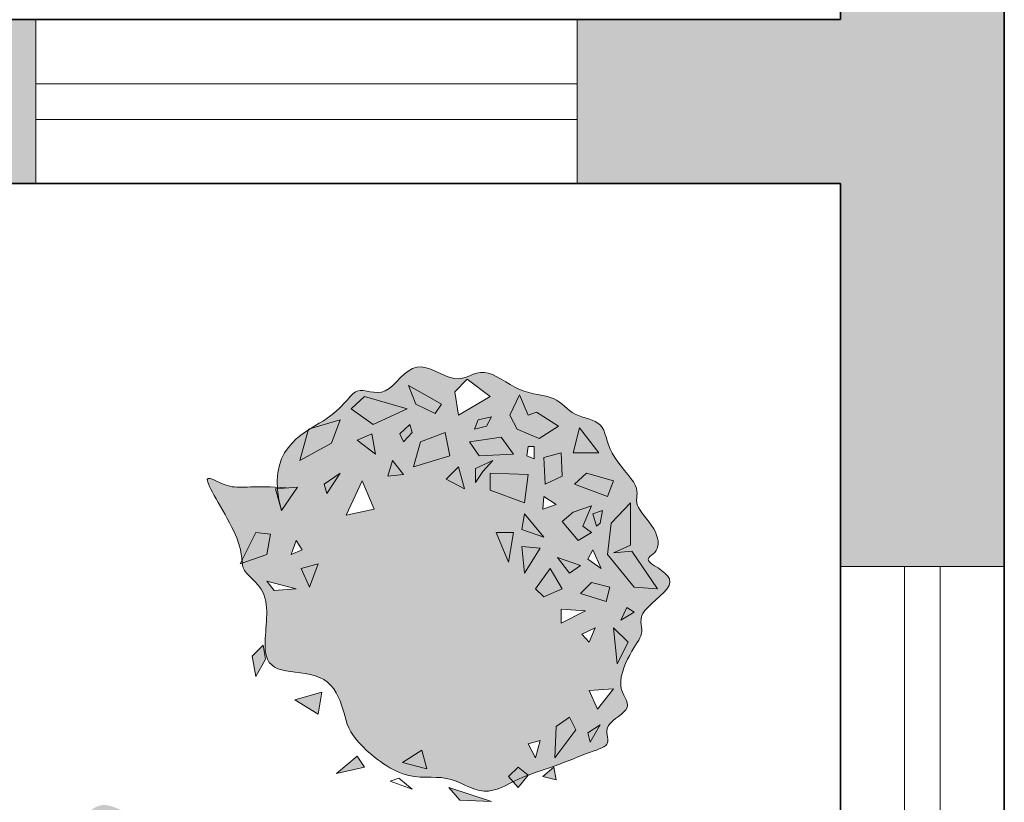
# Model space of a CAD drawing. Units: metres. Extents: x 4298.5 to 4325.2, y 2075 to 2095.8.
# Tile 15 of 35: x 4304.5 to 4305.9, y 2083.7 to 2084.8. Entities that reach past the tile are written whole.
import ezdxf

# ---------------------------------------------------------------- set-up
doc = ezdxf.new("R2010")
doc.units = ezdxf.units.M
for name, color, linetype, lineweight in [('A-ANNO-DIMS', 2, 'Continuous', 18), ('A-GLAZ', 4, 'Continuous', 18), ('A-WALL', 7, 'Continuous', 35), ('A-WALL-PATT', 252, 'Continuous', 13), ('L-PLNT', 94, 'Continuous', 13)]:
    doc.layers.add(name, color=color, linetype=linetype, lineweight=lineweight)
doc.layers.add('L-PLNT-PATT', color=116, linetype='Continuous', lineweight=13, true_color=0x13823e)
doc.styles.get("Standard").update_dxf_attribs({"font": 'arial.ttf'})
doc.dimstyles.get("Standard").update_dxf_attribs({"dimtxt": 0.18, "dimasz": 0.18, "dimexe": 0.18, "dimexo": 0.0625, "dimgap": 0.09, "dimtad": 0, "dimtih": 1, "dimtoh": 1, "dimdec": 4, "dimzin": 0, "dimdsep": 46, "dimtxsty": 'Standard', "dimcen": 0.09, "dimadec": 0, "dimazin": 0, "dimtfac": 1, "dimtdec": 4, "dimtofl": 0, "dimtmove": 0, "dimatfit": 3, "dimfxl": 1, "dimtolj": 1, "dimtzin": 0, "dimarcsym": 0})

# ---------------------------------------------------------------- blocks, each defined once
blk = doc.blocks.new('*U9')
for points in [[(1.237, 12.003), (0.562, 11.31), (0.764, 10.013), (2.519, 11.051)], [(-2.003, 11.656), (-1.598, 10.618), (-0.518, 10.099), (-0.181, 10.618), (-0.788, 10.964)], [(-4.432, 11.051), (-5.175, 10.359), (-3.96, 9.493), (-2.07, 10.359)], [(4.139, 11.137), (3.599, 10.013), (4.004, 9.234), (5.218, 8.715), (6.298, 9.407), (5.083, 10.186), (4.611, 10.013)], [(2.586, 9.926), (1.844, 9.753), (1.642, 9.234), (2.316, 9.407)], [(-5.782, 9.753), (-7.537, 9.234), (-8.009, 7.504), (-6.255, 8.455)], [(-1.935, 9.493), (-2.475, 8.974), (-2.273, 8.542), (-1.8, 9.061)], [(7.446, 9.32), (7.108, 7.936), (8.525, 7.936)], [(-4.837, 8.628), (-3.825, 7.85), (-4.027, 8.974)], [(0.022, 9.061), (-1.328, 8.542), (-1.733, 7.157), (0.292, 7.763)], [(1.372, 8.542), (3.126, 8.801), (3.801, 7.85), (1.912, 7.763)], [(4.611, 8.282), (4.544, 7.763), (4.949, 7.59), (4.949, 8.282)], [(6.433, 7.936), (5.488, 7.676), (5.556, 6.206), (6.501, 6.638)], [(-2.88, 7.504), (-3.15, 6.638), (-2.273, 6.725)], [(0.764, 7.157), (0.089, 6.465), (1.102, 5.946)], [(1.709, 6.292), (1.709, 7.071), (2.654, 7.504), (2.114, 6.898)], [(-5.782, 6.811), (-6.659, 6.206), (-6.524, 5.687)], [(2.519, 6.811), (2.519, 5.86), (4.409, 5.167), (4.611, 6.725)], [(7.851, 6.811), (7.176, 6.206), (8.998, 5.514), (9.335, 6.379)], [(-8.144, 6.033), (-9.359, 5.946), (-9.022, 4.735)], [(-4.567, 6.379), (-5.445, 4.475), (-3.892, 4.821)], [(5.488, 5.514), (5.421, 4.821), (6.163, 5.081)], [(8.12, 4.994), (7.108, 4.648), (6.501, 4.129), (7.378, 3.091), (8.12, 3.524), (7.648, 3.87)], [(10.28, 5.167), (9.2, 4.043), (8.998, 2.312), (10.482, 0.495), (11.765, 0.409), (10.348, 2.485), (9.335, 2.399), (10.28, 2.831)], [(4.409, 4.562), (4.274, 3.697), (5.488, 3.264)], [(8.728, 4.735), (8.188, 4.562), (8.39, 3.87), (8.593, 4.043)], [(-11.316, 1.793), (-9.831, 2.312), (-9.629, 3.437), (-10.439, 3.524)], [(3.531, 1.88), (2.856, 3.524), (3.801, 3.524)], [(-8.212, 3.091), (-8.482, 2.312), (-7.874, 2.572)], [(4.274, 2.745), (5.286, 2.658), (4.409, 1.274)], [(8.188, 2.572), (7.918, 2.053), (8.66, 1.534)], [(-6.997, 1.793), (-7.942, 1.534), (-7.469, 0.495)], [(7.513, 1.707), (6.906, 1.274), (6.231, 2.139)], [(5.826, 1.534), (5.016, 0.409), (5.488, -0.024), (6.501, 0.409)], [(-8.212, 0.409), (-9.426, 0.322), (-9.831, 0.841)], [(8.12, 0.755), (7.513, 0.149), (8.93, -0.283), (9.133, 0.495)], [(7.783, -0.803), (6.433, -1.495), (6.433, -0.716)], [(10.078, -0.629), (9.74, -1.322), (10.482, -0.889)], [(8.323, -1.754), (7.985, -2.533), (7.581, -2.1)], [(9.335, -1.754), (9.538, -3.744), (10.145, -2.533)], [(-10.034, -2.706), (-10.641, -3.312), (-10.439, -4.436), (-9.899, -3.485)], [(-8.279, -5.734), (-6.794, -5.302), (-6.997, -6.513)], [(9.335, -5.129), (8.458, -6.253), (7.985, -5.215)], [(6.096, -8.935), (6.163, -7.205), (6.906, -6.686), (7.243, -7.378)], [(8.053, -8.07), (8.593, -7.118), (7.918, -7.551)], [(5.286, -7.984), (4.611, -8.157), (5.016, -8.935)], [(-2.34, -9.195), (-1.26, -8.503), (-0.99, -9.541)], [(-4.837, -8.849), (-4.432, -9.454), (-5.985, -9.801)], [(4.071, -9.454), (3.531, -9.974), (4.071, -10.579), (4.611, -9.887)], [(6.028, -9.454), (5.421, -9.974), (6.163, -10.147)], [(-2.543, -10.06), (-3.015, -10.233), (-1.8, -10.666)], [(0.224, -10.579), (0.832, -11.272), (2.586, -11.358)]]:
    blk.add_lwpolyline(points, close=True)
blk = doc.blocks.new('WIN-760-GLASS')
for p, q in [((0, 0.76), (0, 0)), ((0.05, 0.76), (0.05, 0))]:
    blk.add_line(p, q)
blk = doc.blocks.new('*D47')
at = {"layer": 'A-ANNO-DIMS', "color": 0, "lineweight": -2, "transparency": 16777216}
for p, q in [((4300.4306, 2084.4956), (4300.4306, 2074.9896)), ((4322.8106, 2084.4956), (4322.8106, 2074.9896)), ((4300.6106, 2075.1696), (4311.2252, 2075.1696)), ((4322.6306, 2075.1696), (4312.016, 2075.1696))]:
    blk.add_line(p, q, dxfattribs=at)
at = {"layer": 'A-ANNO-DIMS', "color": 0, "transparency": 16777216}
for points in [[(4300.6106, 2075.1996), (4300.6106, 2075.1396), (4300.4306, 2075.1696)], [(4322.6306, 2075.1996), (4322.6306, 2075.1396), (4322.8106, 2075.1696)]]:
    blk.add_solid(points, dxfattribs=at)
at = {"layer": 'Defpoints', "color": 0, "transparency": 16777216}
for p in [(4300.4306, 2084.5581), (4322.8106, 2084.5581), (4322.8106, 2075.1696)]:
    blk.add_point(p, dxfattribs=at)
at = {"layer": 'A-ANNO-DIMS', "color": 0, "transparency": 16777216, "insert": (4311.6206, 2075.1696), "char_height": 0.18, "attachment_point": 5}
blk.add_mtext('\\A1;22.38', dxfattribs=at)
blk = doc.blocks.new('*D51')
at = {"layer": 'A-ANNO-DIMS', "color": 0, "lineweight": -2, "transparency": 16777216}
for p, q in [((4305.5981, 2084.5581), (4299.0921, 2084.5581)), ((4299.2721, 2084.3781), (4299.2721, 2082.375)), ((4299.2721, 2080.0081), (4299.2721, 2082.0111)), ((4305.5981, 2079.8281), (4299.0921, 2079.8281))]:
    blk.add_line(p, q, dxfattribs=at)
at = {"layer": 'A-ANNO-DIMS', "color": 0, "transparency": 16777216}
for points in [[(4299.2421, 2084.3781), (4299.3021, 2084.3781), (4299.2721, 2084.5581)], [(4299.2421, 2080.0081), (4299.3021, 2080.0081), (4299.2721, 2079.8281)]]:
    blk.add_solid(points, dxfattribs=at)
at = {"layer": 'Defpoints', "color": 0, "transparency": 16777216}
for p in [(4305.6606, 2084.5581), (4299.2721, 2079.8281), (4305.6606, 2079.8281)]:
    blk.add_point(p, dxfattribs=at)
at = {"layer": 'A-ANNO-DIMS', "color": 0, "transparency": 16777216, "insert": (4299.2721, 2082.1931), "char_height": 0.18, "attachment_point": 5}
blk.add_mtext('\\A1;4.73', dxfattribs=at)
blk = doc.blocks.new('*D56')
at = {"layer": 'A-ANNO-DIMS', "color": 0, "lineweight": -2, "transparency": 16777216}
for p, q in [((4305.8281, 2085.0581), (4299.0921, 2085.0581)), ((4299.2721, 2084.8781), (4299.2721, 2083.74)), ((4299.2721, 2082.2381), (4299.2721, 2083.3761)), ((4305.8281, 2082.0581), (4299.0921, 2082.0581))]:
    blk.add_line(p, q, dxfattribs=at)
at = {"layer": 'A-ANNO-DIMS', "color": 0, "transparency": 16777216}
for points in [[(4299.2421, 2084.8781), (4299.3021, 2084.8781), (4299.2721, 2085.0581)], [(4299.2421, 2082.2381), (4299.3021, 2082.2381), (4299.2721, 2082.0581)]]:
    blk.add_solid(points, dxfattribs=at)
at = {"layer": 'Defpoints', "color": 0, "transparency": 16777216}
for p in [(4299.2721, 2085.0581), (4305.8906, 2085.0581), (4305.8906, 2082.0581)]:
    blk.add_point(p, dxfattribs=at)
at = {"layer": 'A-ANNO-DIMS', "color": 0, "transparency": 16777216, "insert": (4299.2721, 2083.5581), "char_height": 0.18, "attachment_point": 5}
blk.add_mtext('\\A1;3', dxfattribs=at)

msp = doc.modelspace()

# ---------------------------------------------------------------- hatches: boundary and pattern name
at = {"layer": 'A-WALL-PATT'}
h = msp.add_hatch(color=256, dxfattribs=at)
h.dxf.hatch_style = 1
h.paths.add_polyline_path([(4308.7606, 2094.4781), (4308.1606, 2094.4781), (4307.4606, 2094.4781), (4307.4606, 2094.2481), (4308.2706, 2094.2481), (4308.2706, 2094.1281), (4308.3906, 2094.1281), (4308.3906, 2094.2481), (4308.7606, 2094.2481)])
h.paths.add_polyline_path([(4310.1206, 2094.4781), (4309.5206, 2094.4781), (4309.5206, 2094.2481), (4309.8906, 2094.2481), (4309.8906, 2092.2481), (4308.3906, 2092.2481), (4308.3906, 2093.4281), (4308.2706, 2093.4281), (4308.2706, 2092.0181), (4309.8906, 2092.0181), (4309.8906, 2087.0181), (4309.7706, 2087.0181), (4309.7706, 2086.7881), (4309.8906, 2086.7881), (4311.9406, 2086.7881), (4311.9406, 2087.0181), (4310.1206, 2087.0181), (4310.1206, 2089.0181), (4310.2406, 2089.0181), (4310.2406, 2089.1381), (4310.1206, 2089.1381), (4310.1206, 2092.0181), (4310.3078, 2092.0181), (4310.3078, 2092.2481), (4310.1206, 2092.2481)])
h.paths.add_polyline_path([(4311.7406, 2092.2481), (4311.0678, 2092.2481), (4311.0678, 2092.0181), (4311.7406, 2092.0181)], flags=17)
h.paths.add_polyline_path([(4313.1733, 2092.2481), (4312.5006, 2092.2481), (4312.5006, 2092.0181), (4313.1733, 2092.0181)])
h.paths.add_polyline_path([(4314.5378, 2092.2481), (4314.1206, 2092.2481), (4313.9333, 2092.2481), (4313.9333, 2092.0181), (4314.1206, 2092.0181), (4314.1206, 2087.0181), (4314.0006, 2087.0181), (4314.0006, 2086.7881), (4314.1206, 2086.7881), (4315.5718, 2086.7881), (4315.5718, 2087.0181), (4314.3506, 2087.0181), (4314.3506, 2092.0181), (4314.5378, 2092.0181)])
h.paths.add_polyline_path([(4315.9706, 2092.2481), (4315.2978, 2092.2481), (4315.2978, 2092.0181), (4315.9706, 2092.0181)])
h.paths.add_polyline_path([(4317.4033, 2092.2481), (4316.7306, 2092.2481), (4316.7306, 2092.0181), (4317.4033, 2092.0181)])
h.paths.add_polyline_path([(4318.9506, 2092.2481), (4318.3506, 2092.2481), (4318.1633, 2092.2481), (4318.1633, 2092.0181), (4318.3506, 2092.0181), (4318.3506, 2091.8981), (4318.5806, 2091.8981), (4318.5806, 2092.0181), (4318.9506, 2092.0181)])
h.paths.add_polyline_path([(4321.0106, 2092.2481), (4319.7106, 2092.2481), (4319.7106, 2092.0181), (4320.0806, 2092.0181), (4320.0806, 2090.0181), (4318.5806, 2090.0181), (4318.5806, 2091.1981), (4318.3506, 2091.1981), (4318.3506, 2090.0181), (4318.3506, 2087.0181), (4318.2306, 2087.0181), (4318.2306, 2086.7881), (4318.3506, 2086.7881), (4318.3506, 2086.3081), (4318.5806, 2086.3081), (4318.5806, 2089.7881), (4321.7806, 2089.7881), (4321.7806, 2090.0181), (4320.2006, 2090.0181), (4320.2006, 2092.0181), (4321.0106, 2092.0181)])
h.paths.add_polyline_path([(4322.8106, 2092.2481), (4321.7706, 2092.2481), (4321.7706, 2092.0181), (4322.5806, 2092.0181), (4322.5806, 2091.2831), (4322.8106, 2091.2831)])
h.paths.add_polyline_path([(4322.8106, 2090.5231), (4322.5806, 2090.5231), (4322.5806, 2089.7881), (4322.5806, 2089.5254), (4322.8106, 2089.5254), (4322.8106, 2090.0181)])
h.paths.add_polyline_path([(4322.8106, 2088.7654), (4322.5806, 2088.7654), (4322.5806, 2087.6681), (4322.8106, 2087.6681)])
h.paths.add_polyline_path([(4322.8106, 2086.9081), (4322.5806, 2086.9081), (4322.5806, 2085.8107), (4322.8106, 2085.8107)])
h.paths.add_polyline_path([(4322.8106, 2085.0507), (4322.5806, 2085.0507), (4322.5806, 2084.7881), (4318.5806, 2084.7881), (4318.5806, 2085.0581), (4318.5806, 2085.4081), (4318.3506, 2085.4081), (4318.3506, 2084.5581), (4318.3506, 2080.8581), (4318.4706, 2080.8581), (4318.4706, 2082.3281), (4319.2606, 2082.3281), (4319.2606, 2082.5581), (4318.5806, 2082.5581), (4318.5806, 2084.5581), (4320.0806, 2084.5581), (4320.0806, 2083.9381), (4320.3106, 2083.9381), (4320.3106, 2084.5581), (4322.8106, 2084.5581)])
h.paths.add_polyline_path([(4320.3106, 2083.1781), (4320.0806, 2083.1781), (4320.0806, 2082.5581), (4319.9606, 2082.5581), (4319.9606, 2082.3281), (4320.0806, 2082.3281), (4320.0806, 2081.5731), (4320.3106, 2081.5731)], flags=17)
h.paths.add_polyline_path([(4320.3106, 2080.8131), (4320.0806, 2080.8131), (4320.0806, 2080.0581), (4318.4286, 2080.0581), (4318.4286, 2079.8281), (4320.3106, 2079.8281)])
h.paths.add_polyline_path([(4317.3506, 2085.2881), (4316.5718, 2085.2881), (4316.5718, 2085.0581), (4317.3506, 2085.0581)])
h.paths.add_polyline_path([(4315.5718, 2085.2881), (4314.8434, 2085.2881), (4314.8434, 2085.0581), (4315.5718, 2085.0581)])
h.paths.add_polyline_path([(4313.8434, 2085.2881), (4312.9406, 2085.2881), (4312.9406, 2085.0581), (4313.8434, 2085.0581)])
h.paths.add_polyline_path([(4311.9406, 2085.2881), (4311.4406, 2085.2881), (4311.4406, 2085.0581), (4311.9406, 2085.0581)])
h.paths.add_polyline_path([(4317.3306, 2087.0181), (4316.5718, 2087.0181), (4316.5718, 2086.7881), (4317.3306, 2086.7881)])
h.paths.add_polyline_path([(4313.1006, 2089.1381), (4311.1406, 2089.1381), (4311.1406, 2089.0181), (4312.9806, 2089.0181), (4312.9806, 2087.0181), (4312.9406, 2087.0181), (4312.9406, 2086.7881), (4313.1006, 2086.7881), (4313.1006, 2087.0181)])
h.paths.add_polyline_path([(4307.5515, 2087.0181), (4305.8906, 2087.0181), (4305.8906, 2092.2481), (4305.8906, 2094.2481), (4306.7006, 2094.2481), (4306.7006, 2094.4781), (4305.6606, 2094.4781), (4305.6606, 2092.2481), (4305.2906, 2092.2481), (4305.2906, 2092.0181), (4305.6606, 2092.0181), (4305.6606, 2090.0181), (4304.1606, 2090.0181), (4304.1606, 2091.1981), (4304.0406, 2091.1981), (4304.0406, 2089.9081), (4301.5606, 2089.9081), (4301.5606, 2089.7881), (4304.0406, 2089.7881), (4305.6606, 2089.7881), (4305.6606, 2086.6381), (4305.8906, 2086.6381), (4305.8906, 2086.7881), (4307.5515, 2086.7881)])
h.paths.add_polyline_path([(4307.5515, 2085.2881), (4305.8906, 2085.2881), (4305.8906, 2085.4381), (4305.6606, 2085.4381), (4305.6606, 2084.7881), (4305.2906, 2084.7881), (4305.2906, 2084.5581), (4305.6606, 2084.5581), (4305.6606, 2084.02), (4305.8906, 2084.02), (4305.8906, 2084.5581), (4305.8906, 2085.0581), (4307.5515, 2085.0581)])
h.paths.add_polyline_path([(4310.2406, 2085.2881), (4308.5515, 2085.2881), (4308.5515, 2085.0581), (4310.2406, 2085.0581)])
h.paths.add_polyline_path([(4317.4286, 2080.0581), (4316.5718, 2080.0581), (4316.5718, 2079.8281), (4317.4286, 2079.8281)])
h.paths.add_polyline_path([(4315.5718, 2080.0581), (4314.8434, 2080.0581), (4314.8434, 2079.8281), (4315.5718, 2079.8281)])
h.paths.add_polyline_path([(4313.8434, 2080.0581), (4312.9406, 2080.0581), (4312.9406, 2079.8281), (4313.8434, 2079.8281)])
h.paths.add_polyline_path([(4311.9406, 2080.0581), (4311.4406, 2080.0581), (4311.4406, 2079.8281), (4311.9406, 2079.8281)])
h.paths.add_polyline_path([(4310.2406, 2080.0581), (4310.1206, 2080.0581), (4310.1206, 2084.0381), (4309.8906, 2084.0381), (4309.8906, 2080.0581), (4309.1606, 2080.0581), (4309.1606, 2079.8281), (4310.2406, 2079.8281)])
h.paths.add_polyline_path([(4308.1606, 2080.0581), (4307.5106, 2080.0581), (4307.5106, 2080.1781), (4307.3906, 2080.1781), (4307.3906, 2080.0581), (4305.8906, 2080.0581), (4305.8906, 2080.567), (4305.6606, 2080.567), (4305.6606, 2079.8281), (4308.1606, 2079.8281)])
h.paths.add_polyline_path([(4307.5106, 2081.9381), (4309.0906, 2081.9381), (4309.0906, 2082.0581), (4305.8906, 2082.0581), (4305.8906, 2083.26), (4305.6606, 2083.26), (4305.6606, 2081.327), (4305.8906, 2081.327), (4305.8906, 2081.9381), (4307.3906, 2081.9381), (4307.3906, 2080.8781), (4307.5106, 2080.8781)])
h.paths.add_polyline_path([(4304.5306, 2084.7881), (4302.7306, 2084.7881), (4302.7306, 2084.5581), (4304.5306, 2084.5581)])
h.paths.add_polyline_path([(4301.9706, 2084.7881), (4300.6606, 2084.7881), (4300.6606, 2085.0249), (4300.4306, 2085.0249), (4300.4306, 2084.5581), (4301.9706, 2084.5581)])
h.paths.add_polyline_path([(4300.6606, 2086.8843), (4300.4306, 2086.8843), (4300.4306, 2085.7849), (4300.6606, 2085.7849)])
h.paths.add_polyline_path([(4300.6606, 2089.1618), (4300.4306, 2089.1618), (4300.4306, 2087.6443), (4300.6606, 2087.6443)])
h.paths.add_polyline_path([(4300.6606, 2091.0212), (4300.4306, 2091.0212), (4300.4306, 2089.9218), (4300.6606, 2089.9218)])
h.paths.add_polyline_path([(4300.6606, 2092.0181), (4301.9706, 2092.0181), (4301.9706, 2092.2481), (4300.4306, 2092.2481), (4300.4306, 2091.7812), (4300.6606, 2091.7812)])
h.paths.add_polyline_path([(4304.5306, 2092.2481), (4302.7306, 2092.2481), (4302.7306, 2092.0181), (4304.0406, 2092.0181), (4304.0406, 2091.8981), (4304.1606, 2091.8981), (4304.1606, 2092.0181), (4304.5306, 2092.0181)], flags=17)
at = {"layer": 'L-PLNT-PATT'}
h = msp.add_hatch(color=256, dxfattribs=at)
h.dxf.hatch_style = 1
edge = h.paths.add_edge_path()
edge.add_spline(control_points=[(4305.2007, 2083.7177), (4305.2032, 2083.7191), (4305.2219, 2083.7284), (4305.2577, 2083.7381), (4305.3122, 2083.7614), (4305.3415, 2083.769), (4305.3228, 2083.7975), (4305.3754, 2083.8217), (4305.3417, 2083.848), (4305.3687, 2083.9077), (4305.3874, 2083.9272), (4305.3708, 2083.9557), (4305.445, 2084.0006), (4305.3751, 2084.0301), (4305.4078, 2084.0378), (4305.4038, 2084.0729), (4305.3657, 2084.1095), (4305.3842, 2084.1289), (4305.3312, 2084.1799), (4305.3312, 2084.2259), (4305.2833, 2084.2293), (4305.2629, 2084.2612), (4305.2097, 2084.2612), (4305.1574, 2084.3065), (4305.1226, 2084.2694), (4305.0619, 2084.3203), (4305.022, 2084.2502), (4304.9774, 2084.2802), (4304.9631, 2084.2408), (4304.9228, 2084.2178), (4304.9164, 2084.2138)], knot_values=[0.818571, 0.818571, 0.818571, 0.818571, 0.97924, 1.97924, 2.97924, 3.97924, 4.97924, 5.97924, 6.97924, 7.97924, 8.97924, 9.97924, 10.97924, 11.97924, 12.97924, 13.97924, 14.97924, 15.97924, 16.97924, 17.97924, 18.97924, 19.97924, 20.97924, 21.97924, 22.97924, 23.97924, 24.97924, 25.97924, 26.97924, 27.16067, 27.16067, 27.16067, 27.16067], degree=3, periodic=0)
edge.add_line((4304.9164, 2084.2138), (4304.9577, 2084.226))
edge.add_line((4304.9577, 2084.226), (4304.9457, 2084.193))
edge.add_line((4304.9457, 2084.193), (4304.9011, 2084.1689))
edge.add_line((4304.9011, 2084.1689), (4304.9127, 2084.2115))
edge.add_spline(control_points=[(4304.9127, 2084.2115), (4304.8901, 2084.1968), (4304.8668, 2084.1759), (4304.8695, 2084.1315)], knot_values=[0.141368, 0.141368, 0.141368, 0.141368, 0.783694, 0.783694, 0.783694, 0.783694], degree=3, periodic=0)
edge.add_spline(control_points=[(4304.8695, 2084.1315), (4304.8735, 2084.1312), (4304.8777, 2084.1309), (4304.8823, 2084.1304)], knot_values=[40.901028, 40.901028, 40.901028, 40.901028, 41, 41, 41, 41], degree=3, periodic=0)
edge.add_line((4304.8823, 2084.1304), (4304.8977, 2084.1315))
edge.add_line((4304.8977, 2084.1315), (4304.8754, 2084.0985))
edge.add_line((4304.8754, 2084.0985), (4304.8668, 2084.1293))
edge.add_line((4304.8668, 2084.1293), (4304.8697, 2084.1295))
edge.add_spline(control_points=[(4304.8697, 2084.1295), (4304.8696, 2084.1302), (4304.8696, 2084.1308), (4304.8695, 2084.1315)], knot_values=[0.13204, 0.13204, 0.13204, 0.13204, 0.141368, 0.141368, 0.141368, 0.141368], degree=3, periodic=0)
edge.add_spline(control_points=[(4304.8695, 2084.1315), (4304.8333, 2084.1338), (4304.8017, 2084.124), (4304.7497, 2084.1659), (4304.8168, 2084.0634), (4304.8191, 2084.0365), (4304.8198, 2084.0291)], knot_values=[37.439141, 37.439141, 37.439141, 37.439141, 38.340169, 39.340169, 40.340169, 40.901028, 40.901028, 40.901028, 40.901028], degree=3, periodic=0)
edge.add_line((4304.8198, 2084.0291), (4304.8394, 2084.0678))
edge.add_line((4304.8394, 2084.0678), (4304.86, 2084.0656))
edge.add_line((4304.86, 2084.0656), (4304.8548, 2084.037))
edge.add_line((4304.8548, 2084.037), (4304.8202, 2084.0249))
edge.add_spline(control_points=[(4304.8202, 2084.0249), (4304.8207, 2084.021), (4304.8238, 2084.0074), (4304.8651, 2083.9865), (4304.8437, 2083.8892), (4304.8759, 2083.8703), (4304.9421, 2083.8703), (4304.9649, 2083.8166), (4304.9684, 2083.7811), (4305.0494, 2083.7151), (4305.1077, 2083.7318), (4305.1581, 2083.6949), (4305.1872, 2083.7109), (4305.2007, 2083.7177)], knot_values=[27.16067, 27.16067, 27.16067, 27.16067, 27.490087, 28.490087, 29.490087, 30.490087, 31.490087, 32.490087, 33.490087, 34.490087, 35.490087, 36.490087, 37.329418, 37.329418, 37.329418, 37.329418], degree=3, periodic=0)
edge.add_line((4305.2007, 2083.7177), (4305.1942, 2083.7249))
edge.add_line((4305.1942, 2083.7249), (4305.208, 2083.7381))
edge.add_line((4305.208, 2083.7381), (4305.2217, 2083.7271))
h.paths.add_polyline_path([(4305.1771, 2084.0678), (4305.2011, 2084.0678), (4305.1942, 2084.026)], flags=16)
h.paths.add_polyline_path([(4305.2131, 2084.048), (4305.2388, 2084.0458), (4305.2165, 2084.0106)], flags=16)
h.paths.add_polyline_path([(4305.0057, 2084.1007), (4304.9662, 2084.0919), (4304.9885, 2084.1403)], flags=16)
h.paths.add_polyline_path([(4305.1325, 2084.1293), (4305.1068, 2084.1425), (4305.124, 2084.1601)], flags=16)
h.paths.add_polyline_path([(4305.2131, 2084.0722), (4305.2165, 2084.0942), (4305.2439, 2084.0612)], flags=16)
h.paths.add_polyline_path([(4305.232, 2083.9887), (4305.2525, 2084.0172), (4305.2697, 2083.9887), (4305.2439, 2083.9777)], flags=16)
h.paths.add_polyline_path([(4305.1685, 2084.1271), (4305.1685, 2084.1513), (4305.2217, 2084.1491), (4305.2165, 2084.1095)], flags=16)
h.paths.add_polyline_path([(4305.148, 2084.1381), (4305.148, 2084.1579), (4305.172, 2084.1689), (4305.1582, 2084.1535)], flags=16)
h.paths.add_polyline_path([(4305.0468, 2084.1491), (4305.0245, 2084.1469), (4305.0314, 2084.1689)], flags=16)
h.paths.add_polyline_path([(4305.0605, 2084.1601), (4305.0708, 2084.1952), (4305.1051, 2084.2084), (4305.112, 2084.1755)], flags=16)
h.paths.add_polyline_path([(4304.9268, 2084.0238), (4304.9148, 2083.9909), (4304.9028, 2084.0172)], flags=16)
h.paths.add_polyline_path([(4305.2628, 2084.0326), (4305.2954, 2084.0216), (4305.28, 2084.0106)], flags=16)
h.paths.add_polyline_path([(4305.2422, 2084.1007), (4305.2439, 2084.1183), (4305.2611, 2084.1073)], flags=16)
h.paths.add_polyline_path([(4305.1531, 2084.1755), (4305.1394, 2084.1952), (4305.1839, 2084.2018), (4305.2011, 2084.1777)], flags=16)
h.paths.add_polyline_path([(4305.2679, 2083.9601), (4305.3022, 2083.9579), (4305.2679, 2083.9403)], flags=16)
h.paths.add_polyline_path([(4304.9045, 2084.0436), (4304.8891, 2084.037), (4304.896, 2084.0568)], flags=16)
h.paths.add_polyline_path([(4305.0074, 2084.1777), (4304.9817, 2084.1974), (4305.0023, 2084.2062)], flags=16)
h.paths.add_polyline_path([(4304.9388, 2084.1227), (4304.9354, 2084.1359), (4304.9577, 2084.1513)], flags=16)
h.paths.add_polyline_path([(4305.0468, 2084.1952), (4305.0417, 2084.2062), (4305.0554, 2084.2194), (4305.0588, 2084.2084)], flags=16)
h.paths.add_polyline_path([(4305.2697, 2084.0832), (4305.2851, 2084.0963), (4305.3108, 2084.1051), (4305.2988, 2084.0766), (4305.3108, 2084.0678), (4305.2919, 2084.0568)], flags=16)
h.paths.add_polyline_path([(4304.896, 2083.9887), (4304.8651, 2083.9865), (4304.8548, 2083.9996)], flags=16)
h.paths.add_polyline_path([(4305.2457, 2084.1359), (4305.2439, 2084.1732), (4305.2679, 2084.1799), (4305.2697, 2084.1469)], flags=16)
h.paths.add_polyline_path([(4305.2954, 2083.9821), (4305.3108, 2083.9975), (4305.3365, 2083.9909), (4305.3314, 2083.9711)], flags=16)
h.paths.add_polyline_path([(4305.22, 2084.1755), (4305.2217, 2084.1886), (4305.2303, 2084.1886), (4305.2303, 2084.1711)], flags=16)
h.paths.add_polyline_path([(4305.1463, 2084.2128), (4305.1514, 2084.226), (4305.1702, 2084.2304), (4305.1634, 2084.2172)], flags=16)
h.paths.add_polyline_path([(4305.3057, 2084.0304), (4305.3125, 2084.0436), (4305.3245, 2084.0172)], flags=16)
h.paths.add_polyline_path([(4305.2971, 2083.9249), (4305.316, 2083.9337), (4305.3074, 2083.9139)], flags=16)
h.paths.add_polyline_path([(4305.0914, 2084.2348), (4305.064, 2084.248), (4305.0537, 2084.2743), (4305.0845, 2084.2568), (4305.0999, 2084.248)], flags=16)
h.paths.add_polyline_path([(4305.124, 2084.2326), (4305.1188, 2084.2656), (4305.136, 2084.2832), (4305.1685, 2084.259)], flags=16)
h.paths.add_polyline_path([(4305.004, 2084.2194), (4304.9731, 2084.2414), (4304.992, 2084.259), (4305.052, 2084.2414)], flags=16)
h.paths.add_polyline_path([(4305.2868, 2084.1359), (4305.304, 2084.1513), (4305.3417, 2084.1403), (4305.3331, 2084.1183)], flags=16)
h.paths.add_polyline_path([(4305.2062, 2084.2128), (4305.196, 2084.2326), (4305.2097, 2084.2612), (4305.2217, 2084.2326), (4305.2337, 2084.237), (4305.2645, 2084.2172), (4305.2371, 2084.1996)], flags=16)
h.paths.add_polyline_path([(4305.3177, 2084.0766), (4305.3125, 2084.0942), (4305.3262, 2084.0985), (4305.3228, 2084.081)], flags=16)
h.paths.add_polyline_path([(4305.3331, 2084.037), (4305.3382, 2084.081), (4305.3657, 2084.1095), (4305.3657, 2084.0502), (4305.3417, 2084.0392), (4305.3674, 2084.0414), (4305.4034, 2083.9887), (4305.3708, 2083.9909)], flags=16)
h.paths.add_polyline_path([(4305.0725, 2083.7623), (4305.0794, 2083.7359), (4305.0451, 2083.7447)], flags=16)
h.paths.add_polyline_path([(4305.2851, 2084.1799), (4305.2937, 2084.215), (4305.3211, 2084.1799)], flags=16)
h.paths.add_polyline_path([(4305.3417, 2083.9337), (4305.3622, 2083.9139), (4305.3468, 2083.8832)], flags=16)
h.paths.add_polyline_path([(4305.3519, 2083.9447), (4305.3605, 2083.9623), (4305.3708, 2083.9557)], flags=16)
h.paths.add_polyline_path([(4305.2217, 2083.7711), (4305.2388, 2083.7755), (4305.232, 2083.7513)], flags=16)
h.paths.add_polyline_path([(4305.3074, 2083.8458), (4305.3417, 2083.848), (4305.3194, 2083.8195)], flags=16)
h.paths.add_polyline_path([(4305.2611, 2083.7953), (4305.28, 2083.8085), (4305.2885, 2083.7909), (4305.2594, 2083.7513)], flags=16)
h.paths.add_polyline_path([(4305.3057, 2083.7865), (4305.3228, 2083.7975), (4305.3091, 2083.7733)], flags=16)
h = msp.add_hatch(color=256, dxfattribs=at)
h.dxf.hatch_style = 1
h.paths.add_polyline_path([(4305.2165, 2084.1095), (4305.2217, 2084.1491), (4305.1685, 2084.1513), (4305.1685, 2084.1271)])
h.paths.add_polyline_path([(4305.2628, 2084.0326), (4305.28, 2084.0106), (4305.2954, 2084.0216)])
h.paths.add_polyline_path([(4305.2439, 2084.1732), (4305.2457, 2084.1359), (4305.2697, 2084.1469), (4305.2679, 2084.1799)])
h.paths.add_polyline_path([(4305.2645, 2084.2172), (4305.2337, 2084.237), (4305.2217, 2084.2326), (4305.2097, 2084.2612), (4305.196, 2084.2326), (4305.2062, 2084.2128), (4305.2371, 2084.1996)])
h.paths.add_polyline_path([(4305.1102, 2083.7096), (4305.1257, 2083.692), (4305.1702, 2083.6898)])
h.paths.add_polyline_path([(4305.0914, 2084.2348), (4305.0999, 2084.248), (4305.0845, 2084.2568), (4305.0537, 2084.2743), (4305.064, 2084.248)])
h.paths.add_polyline_path([(4304.992, 2084.259), (4304.9731, 2084.2414), (4305.004, 2084.2194), (4305.052, 2084.2414)])
h.paths.add_polyline_path([(4305.0708, 2084.1952), (4305.0605, 2084.1601), (4305.112, 2084.1755), (4305.1051, 2084.2084)])
h.paths.add_polyline_path([(4305.0588, 2084.2084), (4305.0554, 2084.2194), (4305.0417, 2084.2062), (4305.0468, 2084.1952)])
h.paths.add_polyline_path([(4305.0314, 2084.1689), (4305.0245, 2084.1469), (4305.0468, 2084.1491)])
h.paths.add_polyline_path([(4305.0074, 2084.1777), (4305.0023, 2084.2062), (4304.9817, 2084.1974)])
h.paths.add_polyline_path([(4304.9131, 2084.2128), (4304.9011, 2084.1689), (4304.9457, 2084.193), (4304.9577, 2084.226)])
h.paths.add_polyline_path([(4304.9577, 2084.1513), (4304.9354, 2084.1359), (4304.9388, 2084.1227)])
h.paths.add_polyline_path([(4304.8668, 2084.1293), (4304.8754, 2084.0985), (4304.8977, 2084.1315)])
h.paths.add_polyline_path([(4304.8171, 2084.0238), (4304.8548, 2084.037), (4304.86, 2084.0656), (4304.8394, 2084.0678)])
h.paths.add_polyline_path([(4304.9268, 2084.0238), (4304.9028, 2084.0172), (4304.9148, 2083.9909)])
h.paths.add_polyline_path([(4304.8531, 2083.8898), (4304.8497, 2083.9095), (4304.8343, 2083.8942), (4304.8394, 2083.8656)])
h.paths.add_polyline_path([(4304.932, 2083.8436), (4304.8943, 2083.8326), (4304.9268, 2083.8128)])
h.paths.add_polyline_path([(4304.9525, 2083.7293), (4304.992, 2083.7381), (4304.9817, 2083.7535)])
h.paths.add_polyline_path([(4305.0725, 2083.7623), (4305.0451, 2083.7447), (4305.0794, 2083.7359)])
h.paths.add_polyline_path([(4305.208, 2083.7381), (4305.1942, 2083.7249), (4305.208, 2083.7096), (4305.2217, 2083.7271)])
h.paths.add_polyline_path([(4305.2885, 2083.7909), (4305.28, 2083.8085), (4305.2611, 2083.7953), (4305.2594, 2083.7513)])
h.paths.add_polyline_path([(4305.2577, 2083.7381), (4305.2422, 2083.7249), (4305.2611, 2083.7205)])
h.paths.add_polyline_path([(4305.3057, 2083.7865), (4305.3091, 2083.7733), (4305.3228, 2083.7975)])
h.paths.add_polyline_path([(4305.3468, 2083.8832), (4305.3622, 2083.9139), (4305.3417, 2083.9337)])
h.paths.add_polyline_path([(4305.232, 2083.9887), (4305.2439, 2083.9777), (4305.2697, 2083.9887), (4305.2525, 2084.0172)])
h.paths.add_polyline_path([(4305.3708, 2083.9909), (4305.4034, 2083.9887), (4305.3674, 2084.0414), (4305.3417, 2084.0392), (4305.3657, 2084.0502), (4305.3657, 2084.1095), (4305.3382, 2084.081), (4305.3331, 2084.037)])
h.paths.add_polyline_path([(4305.3108, 2083.9975), (4305.2954, 2083.9821), (4305.3314, 2083.9711), (4305.3365, 2083.9909)])
h.paths.add_polyline_path([(4305.3708, 2083.9557), (4305.3605, 2083.9623), (4305.3519, 2083.9447)])
h.paths.add_polyline_path([(4305.3108, 2084.1051), (4305.2851, 2084.0963), (4305.2697, 2084.0832), (4305.2919, 2084.0568), (4305.3108, 2084.0678), (4305.2988, 2084.0766)])
h.paths.add_polyline_path([(4305.3125, 2084.0942), (4305.3177, 2084.0766), (4305.3228, 2084.081), (4305.3262, 2084.0985)])
h.paths.add_polyline_path([(4305.3331, 2084.1183), (4305.3417, 2084.1403), (4305.304, 2084.1513), (4305.2868, 2084.1359)])
h.paths.add_polyline_path([(4305.2439, 2084.0612), (4305.2165, 2084.0942), (4305.2131, 2084.0722)])
h.paths.add_polyline_path([(4305.2011, 2084.0678), (4305.1771, 2084.0678), (4305.1942, 2084.026)])
h.paths.add_polyline_path([(4305.2388, 2084.0458), (4305.2131, 2084.048), (4305.2165, 2084.0106)])
h.paths.add_polyline_path([(4305.2011, 2084.1777), (4305.1839, 2084.2018), (4305.1394, 2084.1952), (4305.1531, 2084.1755)])
h.paths.add_polyline_path([(4305.1582, 2084.1535), (4305.172, 2084.1689), (4305.148, 2084.1579), (4305.148, 2084.1381)])
h.paths.add_polyline_path([(4305.124, 2084.1601), (4305.1068, 2084.1425), (4305.1325, 2084.1293)])
h.paths.add_polyline_path([(4305.1634, 2084.2172), (4305.1702, 2084.2304), (4305.1514, 2084.226), (4305.1463, 2084.2128)])
h.paths.add_polyline_path([(4305.2937, 2084.215), (4305.2851, 2084.1799), (4305.3211, 2084.1799)])
h = msp.add_hatch(color=256, dxfattribs=at)
h.dxf.hatch_style = 1
edge = h.paths.add_edge_path()
edge.add_spline(control_points=[(4304.7568, 2083.1024), (4304.7594, 2083.1037), (4304.778, 2083.1131), (4304.8138, 2083.1228), (4304.8683, 2083.1461), (4304.8977, 2083.1537), (4304.8789, 2083.1822), (4304.9315, 2083.2063), (4304.8978, 2083.2327), (4304.9248, 2083.2924), (4304.9435, 2083.3119), (4304.9269, 2083.3404), (4305.0011, 2083.3852), (4304.9312, 2083.4148), (4304.9639, 2083.4224), (4304.9599, 2083.4576), (4304.9218, 2083.4942), (4304.9404, 2083.5135), (4304.8873, 2083.5645), (4304.8873, 2083.6106), (4304.8395, 2083.6139), (4304.819, 2083.6458), (4304.7658, 2083.6458), (4304.7135, 2083.6912), (4304.6787, 2083.6541), (4304.618, 2083.7049), (4304.5781, 2083.6349), (4304.5335, 2083.6648), (4304.5192, 2083.6255), (4304.4789, 2083.6024), (4304.4725, 2083.5985)], knot_values=[0.818571, 0.818571, 0.818571, 0.818571, 0.97924, 1.97924, 2.97924, 3.97924, 4.97924, 5.97924, 6.97924, 7.97924, 8.97924, 9.97924, 10.97924, 11.97924, 12.97924, 13.97924, 14.97924, 15.97924, 16.97924, 17.97924, 18.97924, 19.97924, 20.97924, 21.97924, 22.97924, 23.97924, 24.97924, 25.97924, 26.97924, 27.16067, 27.16067, 27.16067, 27.16067], degree=3, periodic=0)
edge.add_line((4304.4725, 2083.5985), (4304.5138, 2083.6107))
edge.add_line((4304.5138, 2083.6107), (4304.5018, 2083.5777))
edge.add_line((4304.5018, 2083.5777), (4304.4572, 2083.5536))
edge.add_line((4304.4572, 2083.5536), (4304.4689, 2083.5961))
edge.add_spline(control_points=[(4304.4689, 2083.5961), (4304.4462, 2083.5815), (4304.4229, 2083.5605), (4304.4256, 2083.5161)], knot_values=[0.141368, 0.141368, 0.141368, 0.141368, 0.783694, 0.783694, 0.783694, 0.783694], degree=3, periodic=0)
edge.add_spline(control_points=[(4304.4256, 2083.5161), (4304.4296, 2083.5159), (4304.4339, 2083.5155), (4304.4384, 2083.5151)], knot_values=[40.901028, 40.901028, 40.901028, 40.901028, 41, 41, 41, 41], degree=3, periodic=0)
edge.add_line((4304.4384, 2083.5151), (4304.4538, 2083.5162))
edge.add_line((4304.4538, 2083.5162), (4304.4315, 2083.4832))
edge.add_line((4304.4315, 2083.4832), (4304.423, 2083.514))
edge.add_line((4304.423, 2083.514), (4304.4258, 2083.5142))
edge.add_spline(control_points=[(4304.4258, 2083.5142), (4304.4257, 2083.5148), (4304.4257, 2083.5155), (4304.4256, 2083.5161)], knot_values=[0.13204, 0.13204, 0.13204, 0.13204, 0.141368, 0.141368, 0.141368, 0.141368], degree=3, periodic=0)
edge.add_spline(control_points=[(4304.4256, 2083.5161), (4304.3894, 2083.5185), (4304.3578, 2083.5086), (4304.3058, 2083.5506), (4304.3729, 2083.4481), (4304.3752, 2083.4212), (4304.3759, 2083.4137)], knot_values=[37.439141, 37.439141, 37.439141, 37.439141, 38.340169, 39.340169, 40.340169, 40.901028, 40.901028, 40.901028, 40.901028], degree=3, periodic=0)
edge.add_line((4304.3759, 2083.4137), (4304.3955, 2083.4525))
edge.add_line((4304.3955, 2083.4525), (4304.4161, 2083.4502))
edge.add_line((4304.4161, 2083.4502), (4304.411, 2083.4217))
edge.add_line((4304.411, 2083.4217), (4304.3763, 2083.4096))
edge.add_spline(control_points=[(4304.3763, 2083.4096), (4304.3768, 2083.4056), (4304.3799, 2083.3921), (4304.4212, 2083.3711), (4304.3998, 2083.2738), (4304.432, 2083.255), (4304.4983, 2083.255), (4304.521, 2083.2013), (4304.5245, 2083.1658), (4304.6055, 2083.0997), (4304.6638, 2083.1165), (4304.7142, 2083.0796), (4304.7433, 2083.0956), (4304.7568, 2083.1024)], knot_values=[27.16067, 27.16067, 27.16067, 27.16067, 27.490087, 28.490087, 29.490087, 30.490087, 31.490087, 32.490087, 33.490087, 34.490087, 35.490087, 36.490087, 37.329418, 37.329418, 37.329418, 37.329418], degree=3, periodic=0)
edge.add_line((4304.7568, 2083.1024), (4304.7504, 2083.1096))
edge.add_line((4304.7504, 2083.1096), (4304.7641, 2083.1228))
edge.add_line((4304.7641, 2083.1228), (4304.7778, 2083.1118))
h.paths.add_polyline_path([(4304.7332, 2083.4525), (4304.7572, 2083.4525), (4304.7504, 2083.4107)], flags=16)
h.paths.add_polyline_path([(4304.7692, 2083.4327), (4304.7949, 2083.4305), (4304.7727, 2083.3953)], flags=16)
h.paths.add_polyline_path([(4304.5618, 2083.4854), (4304.5224, 2083.4766), (4304.5447, 2083.525)], flags=16)
h.paths.add_polyline_path([(4304.6887, 2083.514), (4304.6629, 2083.5272), (4304.6801, 2083.5447)], flags=16)
h.paths.add_polyline_path([(4304.7692, 2083.4569), (4304.7727, 2083.4788), (4304.8001, 2083.4459)], flags=16)
h.paths.add_polyline_path([(4304.7881, 2083.3733), (4304.8087, 2083.4019), (4304.8258, 2083.3733), (4304.8001, 2083.3623)], flags=16)
h.paths.add_polyline_path([(4304.7247, 2083.5118), (4304.7247, 2083.5359), (4304.7778, 2083.5338), (4304.7727, 2083.4942)], flags=16)
h.paths.add_polyline_path([(4304.7041, 2083.5228), (4304.7041, 2083.5426), (4304.7281, 2083.5536), (4304.7144, 2083.5382)], flags=16)
h.paths.add_polyline_path([(4304.6029, 2083.5338), (4304.5807, 2083.5316), (4304.5875, 2083.5536)], flags=16)
h.paths.add_polyline_path([(4304.6167, 2083.5447), (4304.6269, 2083.5799), (4304.6612, 2083.5931), (4304.6681, 2083.5601)], flags=16)
h.paths.add_polyline_path([(4304.4829, 2083.4085), (4304.471, 2083.3755), (4304.4589, 2083.4019)], flags=16)
h.paths.add_polyline_path([(4304.8189, 2083.4173), (4304.8515, 2083.4063), (4304.8361, 2083.3953)], flags=16)
h.paths.add_polyline_path([(4304.7984, 2083.4854), (4304.8001, 2083.503), (4304.8172, 2083.492)], flags=16)
h.paths.add_polyline_path([(4304.7092, 2083.5601), (4304.6955, 2083.5799), (4304.7401, 2083.5865), (4304.7572, 2083.5623)], flags=16)
h.paths.add_polyline_path([(4304.8241, 2083.3448), (4304.8584, 2083.3426), (4304.8241, 2083.325)], flags=16)
h.paths.add_polyline_path([(4304.4607, 2083.4283), (4304.4452, 2083.4217), (4304.4521, 2083.4415)], flags=16)
h.paths.add_polyline_path([(4304.5635, 2083.5623), (4304.5378, 2083.5821), (4304.5584, 2083.5909)], flags=16)
h.paths.add_polyline_path([(4304.495, 2083.5074), (4304.4915, 2083.5206), (4304.5138, 2083.5359)], flags=16)
h.paths.add_polyline_path([(4304.6029, 2083.5799), (4304.5978, 2083.5909), (4304.6115, 2083.6041), (4304.615, 2083.5931)], flags=16)
h.paths.add_polyline_path([(4304.8258, 2083.4678), (4304.8412, 2083.481), (4304.8669, 2083.4898), (4304.8549, 2083.4612), (4304.8669, 2083.4525), (4304.8481, 2083.4415)], flags=16)
h.paths.add_polyline_path([(4304.4521, 2083.3733), (4304.4212, 2083.3711), (4304.411, 2083.3843)], flags=16)
h.paths.add_polyline_path([(4304.8018, 2083.5206), (4304.8001, 2083.5579), (4304.8241, 2083.5645), (4304.8258, 2083.5316)], flags=16)
h.paths.add_polyline_path([(4304.8515, 2083.3667), (4304.8669, 2083.3821), (4304.8926, 2083.3755), (4304.8875, 2083.3558)], flags=16)
h.paths.add_polyline_path([(4304.7761, 2083.5601), (4304.7778, 2083.5733), (4304.7864, 2083.5733), (4304.7864, 2083.5557)], flags=16)
h.paths.add_polyline_path([(4304.7024, 2083.5975), (4304.7075, 2083.6107), (4304.7264, 2083.6151), (4304.7195, 2083.6019)], flags=16)
h.paths.add_polyline_path([(4304.8618, 2083.4151), (4304.8686, 2083.4283), (4304.8806, 2083.4019)], flags=16)
h.paths.add_polyline_path([(4304.8532, 2083.3096), (4304.8721, 2083.3184), (4304.8635, 2083.2986)], flags=16)
h.paths.add_polyline_path([(4304.6475, 2083.6195), (4304.6201, 2083.6326), (4304.6098, 2083.659), (4304.6407, 2083.6414), (4304.6561, 2083.6326)], flags=16)
h.paths.add_polyline_path([(4304.6801, 2083.6173), (4304.6749, 2083.6502), (4304.6921, 2083.6678), (4304.7247, 2083.6436)], flags=16)
h.paths.add_polyline_path([(4304.5601, 2083.6041), (4304.5292, 2083.6261), (4304.5481, 2083.6436), (4304.6081, 2083.6261)], flags=16)
h.paths.add_polyline_path([(4304.8429, 2083.5206), (4304.8601, 2083.5359), (4304.8978, 2083.525), (4304.8892, 2083.503)], flags=16)
h.paths.add_polyline_path([(4304.7624, 2083.5975), (4304.7521, 2083.6173), (4304.7658, 2083.6458), (4304.7778, 2083.6173), (4304.7898, 2083.6217), (4304.8206, 2083.6019), (4304.7932, 2083.5843)], flags=16)
h.paths.add_polyline_path([(4304.8738, 2083.4612), (4304.8686, 2083.4788), (4304.8824, 2083.4832), (4304.8789, 2083.4656)], flags=16)
h.paths.add_polyline_path([(4304.8892, 2083.4217), (4304.8944, 2083.4656), (4304.9218, 2083.4942), (4304.9218, 2083.4349), (4304.8978, 2083.4239), (4304.9235, 2083.4261), (4304.9595, 2083.3733), (4304.9269, 2083.3755)], flags=16)
h.paths.add_polyline_path([(4304.6287, 2083.147), (4304.6355, 2083.1206), (4304.6012, 2083.1294)], flags=16)
h.paths.add_polyline_path([(4304.8412, 2083.5645), (4304.8498, 2083.5997), (4304.8772, 2083.5645)], flags=16)
h.paths.add_polyline_path([(4304.8978, 2083.3184), (4304.9184, 2083.2986), (4304.9029, 2083.2679)], flags=16)
h.paths.add_polyline_path([(4304.9081, 2083.3294), (4304.9167, 2083.347), (4304.9269, 2083.3404)], flags=16)
h.paths.add_polyline_path([(4304.7778, 2083.1558), (4304.7949, 2083.1602), (4304.7881, 2083.136)], flags=16)
h.paths.add_polyline_path([(4304.8635, 2083.2305), (4304.8978, 2083.2327), (4304.8755, 2083.2041)], flags=16)
h.paths.add_polyline_path([(4304.8172, 2083.1799), (4304.8361, 2083.1931), (4304.8446, 2083.1755), (4304.8155, 2083.136)], flags=16)
h.paths.add_polyline_path([(4304.8618, 2083.1712), (4304.8789, 2083.1822), (4304.8652, 2083.158)], flags=16)

# ---------------------------------------------------------------- linework, layer by layer
at = {"layer": 'A-GLAZ'}
for p, q in [((4304.5306, 2084.5581), (4304.5306, 2084.7881)), ((4305.2906, 2084.5581), (4305.2906, 2084.7881)), ((4305.6606, 2084.02), (4305.8906, 2084.02))]:
    msp.add_line(p, q, dxfattribs=at)
at = {"layer": 'A-WALL'}
for p, q in [((4305.6606, 2085.4631), (4305.6606, 2084.7881)), ((4305.8906, 2085.0581), (4305.8906, 2084.5581)), ((4305.6606, 2084.7881), (4300.6606, 2084.7881)), ((4305.6606, 2084.5581), (4300.4306, 2084.5581)), ((4305.6606, 2084.5581), (4305.6606, 2079.8281)), ((4305.8906, 2084.5581), (4305.8906, 2082.0581))]:
    msp.add_line(p, q, dxfattribs=at)
at = {"layer": 'L-PLNT'}
msp.add_open_spline([(4304.8754, 2084.0985), (4304.8513, 2084.1851), (4304.9577, 2084.226), (4304.9774, 2084.2802), (4305.022, 2084.2502), (4305.0619, 2084.3203), (4305.1226, 2084.2694), (4305.1574, 2084.3065), (4305.2097, 2084.2612), (4305.2629, 2084.2612), (4305.2833, 2084.2293), (4305.3312, 2084.2259), (4305.3312, 2084.1799), (4305.3842, 2084.1289), (4305.3657, 2084.1095), (4305.4038, 2084.0729), (4305.4078, 2084.0378), (4305.3751, 2084.0301), (4305.445, 2084.0006), (4305.3708, 2083.9557), (4305.3874, 2083.9272), (4305.3687, 2083.9077), (4305.3417, 2083.848), (4305.3754, 2083.8217), (4305.3228, 2083.7975), (4305.3415, 2083.769), (4305.3122, 2083.7614), (4305.2577, 2083.7381), (4305.208, 2083.7246), (4305.1609, 2083.6929), (4305.1077, 2083.7318), (4305.0494, 2083.7151), (4304.9684, 2083.7811), (4304.9649, 2083.8166), (4304.9421, 2083.8703), (4304.8759, 2083.8703), (4304.8437, 2083.8892), (4304.8651, 2083.9865), (4304.8119, 2084.0134), (4304.8283, 2084.0458), (4304.7497, 2084.1659), (4304.8035, 2084.1225), (4304.8366, 2084.1349), (4304.8823, 2084.1304)], degree=3, dxfattribs=at)

# ---------------------------------------------------------------- block references
at = {"layer": 'A-GLAZ'}
for p, rotation in [((4304.5306, 2084.6981), 269.9999999999362), ((4305.8006, 2084.02), 180)]:
    msp.add_blockref('WIN-760-GLASS', p, dxfattribs=dict(at, rotation=rotation))
at = {"layer": 'L-PLNT', "xscale": 0.0254, "yscale": 0.0254, "zscale": 0.0254}
msp.add_blockref('*U9', (4305.1046, 2083.9783), dxfattribs=at)

# ---------------------------------------------------------------- dimensions: what is measured, and where the dimension line sits
at = {"layer": 'A-ANNO-DIMS'}
for base, p1, p2, override, picture, middle in [((4299.2721, 2085.0581), (4305.8906, 2082.0581), (4305.8906, 2085.0581), {"dimdec": 0, "dimlfac": 1, "dimrnd": 0, "dimzin": 0, "dimdsep": 46, "dimlunit": 2}, '*D56', (4299.2721, 2083.5581)), ((4299.2721, 2079.8281), (4305.6606, 2084.5581), (4305.6606, 2079.8281), {"dimdec": 2, "dimlfac": 1, "dimrnd": 0, "dimzin": 0, "dimdsep": 46, "dimlunit": 2}, '*D51', (4299.2721, 2082.1931))]:
    dim = msp.add_linear_dim(base=base, p1=p1, p2=p2, angle=90, dimstyle='Standard', override=override, dxfattribs=at)
    dim.commit()
    dim.dimension.update_dxf_attribs({"geometry": picture, "text_midpoint": middle})
dim = msp.add_linear_dim(base=(4322.8106, 2075.1696), p1=(4300.4306, 2084.5581), p2=(4322.8106, 2084.5581), dimstyle='Standard', override={"dimdec": 2, "dimlfac": 1, "dimrnd": 0, "dimzin": 0, "dimdsep": 46, "dimlunit": 2}, dxfattribs=at)
dim.commit()
dim.dimension.update_dxf_attribs({"geometry": '*D47', "text_midpoint": (4311.6206, 2075.1696)})

doc.saveas('drawing.dxf')
